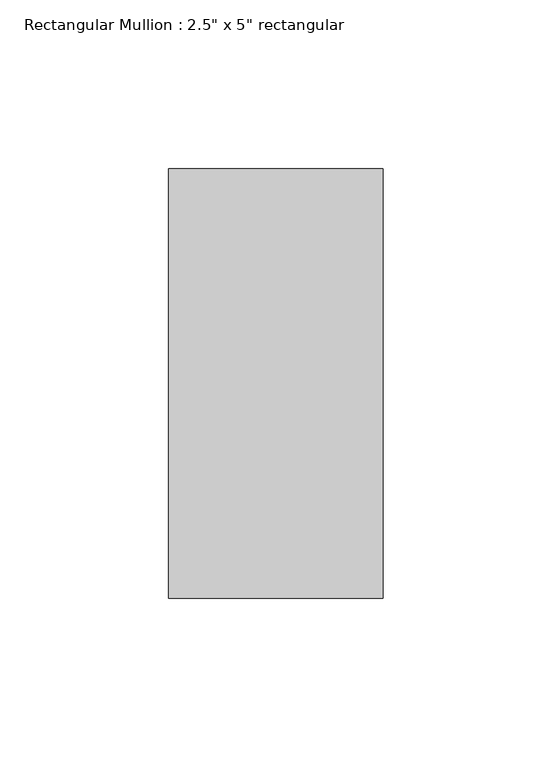
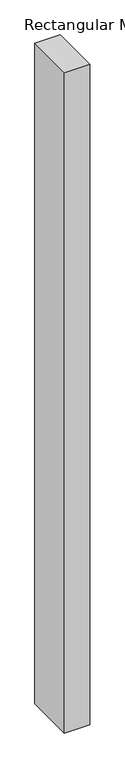
"""IFC4 building model written with IfcOpenShell, lengths in millimetres: member geometry."""

from ifc_helpers import new_model, si_unit, frame, origin, place, context, project, spatial, polyline, outline, extrude, source, transform, mapped, element, save


def member_876c57a8(model_context):
    return source(origin(), model_context, "Body", "SweptSolid", [
        extrude(outline(polyline([(0.0, 63.5), (0.0, -63.5), (-63.5, -63.5), (-63.5, 63.5), (0.0, 63.5)])), frame((0.0, 0.0, -1736.0162259), z_axis=(0.0, 0.0, 1.0), x_axis=(1.0, 0.0, 0.0)), (0.0, 0.0, 1.0), 1736.0162259),
    ])


if __name__ == "__main__":
    model = new_model("IFC4")
    model_context = context("Model", 3, world=origin())
    ifc_project = project(units=[si_unit("LENGTHUNIT", "METRE", prefix="MILLI")], contexts=[model_context])
    site = spatial("IfcSite", under=ifc_project)
    building = spatial("IfcBuilding", under=site)
    placement = place(None, origin())
    member_shape = member_876c57a8(model_context)
    element("IfcMember", 1, ObjectType="Rectangular Mullion : 2.5\" x 5\" rectangular", at=placement, inside=building, context=model_context, shape_type="MappedRepresentation", body=[
        mapped(member_shape, transform((0.0, 0.0, 0.0), x_axis=(1.0, 0.0, 0.0), y_axis=(0.0, 1.0, 0.0), z_axis=(0.0, 0.0, 1.0))),
    ])
    save(model, "model.ifc")

# Revit data of these elements
# Type "Rectangular Mullion : 2.5\" x 5\" rectangular"
#   built-in parameter 1007304 = 0.416667 (stored number, unit not read)
#   built-in parameter 1007301 = 0.104167 (stored number, unit not read)
#   built-in parameter 1007300 = 0.104167 (stored number, unit not read)
# Element 1 (IfcMember, "Rectangular Mullion : 2.5\" x 5\" rectangular")
#   Materials on its faces: "Aluminum"
# Materials
#   "Aluminum": class "Metal", colour RGB 247 247 247, transparency 0, Description = "Aluminum 6061", Cost = 0
